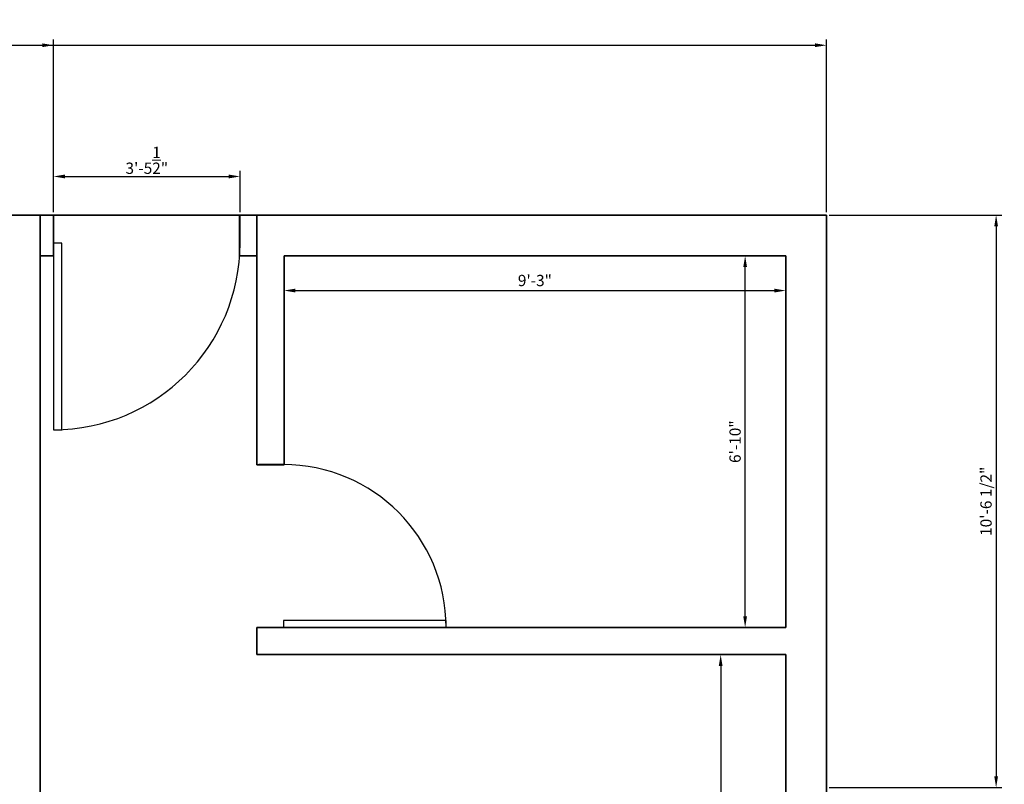
# Model space of a CAD drawing. Units: inches. Extents: x 2025 to 2528, y 1525 to 2336.
# Tile 18 of 18: x 2311 to 2528, y 2167 to 2336. Entities that reach past the tile are written whole.
import ezdxf

# ---------------------------------------------------------------- set-up
doc = ezdxf.new("R2010")
doc.units = ezdxf.units.IN
for name, color, linetype, lineweight in [('A-ANNO-DIMS', 2, 'Continuous', 18), ('A-DOOR', 3, 'Continuous', 25), ('A-WALL', 7, 'Continuous', 35)]:
    doc.layers.add(name, color=color, linetype=linetype, lineweight=lineweight)
doc.styles.get("Standard").update_dxf_attribs({"font": 'arial.ttf'})
doc.dimstyles.new('Copy of ISO-25', dxfattribs={"dimtxt": 2.5, "dimasz": 2.5, "dimexe": 1.25, "dimexo": 0.625, "dimtad": 1, "dimdec": 1, "dimlunit": 4, "dimtxsty": 'Standard', "dimcen": 2.5, "dimadec": 0, "dimazin": 0, "dimtfac": 1, "dimtdec": 1, "dimtmove": 0, "dimatfit": 3, "dimfxl": 1, "dimarcsym": 0})

# ---------------------------------------------------------------- blocks, each defined once
blk = doc.blocks.new('*U2')
for p, q in [((0, 0), (0, 6)), ((40, 0), (40, 6))]:
    blk.add_line(p, q)
blk.add_lwpolyline([(0, 0), (0, -40), (1.75, -40), (1.75, 0)], close=True)
blk.add_arc((0, 0), 40, 270, 0)
blk = doc.blocks.new('*D16')
at = {"layer": 'A-ANNO-DIMS', "color": 0, "lineweight": -2, "transparency": 16777216}
for p, q in [((2369.01, 2282.79), (2369.01, 2274.47)), ((2480.01, 2282.79), (2480.01, 2274.47)), ((2371.51, 2275.72), (2477.51, 2275.72))]:
    blk.add_line(p, q, dxfattribs=at)
at = {"layer": 'A-ANNO-DIMS', "color": 0, "transparency": 16777216}
for points in [[(2371.51, 2276.14), (2371.51, 2275.3), (2369.01, 2275.72)], [(2477.51, 2276.14), (2477.51, 2275.3), (2480.01, 2275.72)]]:
    blk.add_solid(points, dxfattribs=at)
at = {"layer": 'Defpoints', "color": 0, "transparency": 16777216}
for p in [(2369.01, 2283.41), (2480.01, 2283.41), (2480.01, 2275.72)]:
    blk.add_point(p, dxfattribs=at)
at = {"layer": 'A-ANNO-DIMS', "color": 0, "transparency": 16777216, "insert": (2424.51, 2277.62), "char_height": 2.5, "attachment_point": 5}
blk.add_mtext('9\'-3"', dxfattribs=at)
blk = doc.blocks.new('*D17')
at = {"layer": 'A-ANNO-DIMS', "color": 0, "lineweight": -2, "transparency": 16777216}
for p, q in [((2479.39, 2283.41), (2469.78, 2283.41)), ((2471.03, 2203.72), (2471.03, 2280.91)), ((2479.39, 2201.22), (2469.78, 2201.22))]:
    blk.add_line(p, q, dxfattribs=at)
at = {"layer": 'A-ANNO-DIMS', "color": 0, "transparency": 16777216}
for points in [[(2470.61, 2280.91), (2471.45, 2280.91), (2471.03, 2283.41)], [(2470.61, 2203.72), (2471.45, 2203.72), (2471.03, 2201.22)]]:
    blk.add_solid(points, dxfattribs=at)
at = {"layer": 'Defpoints', "color": 0, "transparency": 16777216}
for p in [(2471.03, 2283.41), (2480.01, 2283.41), (2480.01, 2201.22)]:
    blk.add_point(p, dxfattribs=at)
at = {"layer": 'A-ANNO-DIMS', "color": 0, "transparency": 16777216, "insert": (2469.13, 2242.31), "char_height": 2.5, "attachment_point": 5, "rotation": 90}
blk.add_mtext('6\'-10"', dxfattribs=at)
blk = doc.blocks.new('*D18')
at = {"layer": 'A-ANNO-DIMS', "color": 0, "lineweight": -2, "transparency": 16777216}
for p, q in [((2479.39, 2195.22), (2464.37, 2195.22)), ((2465.62, 2192.72), (2465.62, 1943.91)), ((2479.39, 1941.41), (2464.37, 1941.41))]:
    blk.add_line(p, q, dxfattribs=at)
at = {"layer": 'A-ANNO-DIMS', "color": 0, "transparency": 16777216}
for points in [[(2465.2, 2192.72), (2466.03, 2192.72), (2465.62, 2195.22)], [(2465.2, 1943.91), (2466.03, 1943.91), (2465.62, 1941.41)]]:
    blk.add_solid(points, dxfattribs=at)
at = {"layer": 'Defpoints', "color": 0, "transparency": 16777216}
for p in [(2480.01, 2195.22), (2465.62, 1941.41), (2480.01, 1941.41)]:
    blk.add_point(p, dxfattribs=at)
at = {"layer": 'A-ANNO-DIMS', "color": 0, "transparency": 16777216, "insert": (2463.74, 2068.31), "char_height": 2.5, "attachment_point": 5, "rotation": 90}
blk.add_mtext('21\'-2"', dxfattribs=at)
blk = doc.blocks.new('*D20')
at = {"layer": 'A-ANNO-DIMS', "color": 0, "lineweight": -2, "transparency": 16777216}
for p, q in [((2318.01, 2293.04), (2318.01, 2302.2)), ((2320.51, 2300.95), (2356.77, 2300.95)), ((2359.27, 2293.04), (2359.27, 2302.2))]:
    blk.add_line(p, q, dxfattribs=at)
at = {"layer": 'A-ANNO-DIMS', "color": 0, "transparency": 16777216}
for points in [[(2320.51, 2301.37), (2320.51, 2300.53), (2318.01, 2300.95)], [(2356.77, 2301.37), (2356.77, 2300.53), (2359.27, 2300.95)]]:
    blk.add_solid(points, dxfattribs=at)
at = {"layer": 'Defpoints', "color": 0, "transparency": 16777216}
for p in [(2359.27, 2300.95), (2318.01, 2292.41), (2359.27, 2292.41)]:
    blk.add_point(p, dxfattribs=at)
at = {"layer": 'A-ANNO-DIMS', "color": 0, "transparency": 16777216, "insert": (2338.64, 2304.52), "char_height": 2.5, "attachment_point": 5}
blk.add_mtext('3\'-5{\\H1x;\\S1/2;}"', dxfattribs=at)
blk = doc.blocks.new('*D62')
at = {"layer": 'A-ANNO-DIMS', "color": 0, "lineweight": -2, "transparency": 16777216}
for p, q in [((2228.48, 2293.04), (2228.48, 2331.21)), ((2318.01, 2293.04), (2318.01, 2331.21)), ((2230.98, 2329.96), (2315.51, 2329.96))]:
    blk.add_line(p, q, dxfattribs=at)
at = {"layer": 'A-ANNO-DIMS', "color": 0, "transparency": 16777216}
for points in [[(2230.98, 2330.38), (2230.98, 2329.55), (2228.48, 2329.96)], [(2315.51, 2330.38), (2315.51, 2329.55), (2318.01, 2329.96)]]:
    blk.add_solid(points, dxfattribs=at)
at = {"layer": 'Defpoints', "color": 0, "transparency": 16777216}
for p in [(2318.01, 2329.96), (2228.48, 2292.41), (2318.01, 2292.41)]:
    blk.add_point(p, dxfattribs=at)
at = {"layer": 'A-ANNO-DIMS', "color": 0, "transparency": 16777216, "insert": (2273.25, 2331.88), "char_height": 2.5, "attachment_point": 5}
blk.add_mtext('7\'-5 1/2"', dxfattribs=at)
blk = doc.blocks.new('*D63')
at = {"layer": 'A-ANNO-DIMS', "color": 0, "lineweight": -2, "transparency": 16777216}
for p, q in [((2489.64, 2292.41), (2527.81, 2292.41)), ((2526.56, 2289.91), (2526.56, 2168.34)), ((2489.64, 2165.84), (2527.81, 2165.84))]:
    blk.add_line(p, q, dxfattribs=at)
at = {"layer": 'A-ANNO-DIMS', "color": 0, "transparency": 16777216}
for points in [[(2526.15, 2289.91), (2526.98, 2289.91), (2526.56, 2292.41)], [(2526.15, 2168.34), (2526.98, 2168.34), (2526.56, 2165.84)]]:
    blk.add_solid(points, dxfattribs=at)
at = {"layer": 'Defpoints', "color": 0, "transparency": 16777216}
for p in [(2489.01, 2292.41), (2489.01, 2165.84), (2526.56, 2165.84)]:
    blk.add_point(p, dxfattribs=at)
at = {"layer": 'A-ANNO-DIMS', "color": 0, "transparency": 16777216, "insert": (2524.65, 2229.13), "char_height": 2.5, "attachment_point": 5, "rotation": 90}
blk.add_mtext('10\'-6 1/2"', dxfattribs=at)
blk = doc.blocks.new('*D79')
at = {"layer": 'A-ANNO-DIMS', "color": 0, "lineweight": -2, "transparency": 16777216}
for p, q in [((2066.01, 2293.04), (2066.01, 2331.21)), ((2489.01, 2293.04), (2489.01, 2331.21)), ((2068.51, 2329.96), (2486.51, 2329.96))]:
    blk.add_line(p, q, dxfattribs=at)
at = {"layer": 'A-ANNO-DIMS', "color": 0, "transparency": 16777216}
for points in [[(2068.51, 2330.38), (2068.51, 2329.55), (2066.01, 2329.96)], [(2486.51, 2330.38), (2486.51, 2329.55), (2489.01, 2329.96)]]:
    blk.add_solid(points, dxfattribs=at)
at = {"layer": 'Defpoints', "color": 0, "transparency": 16777216}
for p in [(2489.01, 2329.96), (2066.01, 2292.41), (2489.01, 2292.41)]:
    blk.add_point(p, dxfattribs=at)
at = {"layer": 'A-ANNO-DIMS', "color": 0, "transparency": 16777216, "insert": (2277.51, 2331.86), "char_height": 2.5, "attachment_point": 5}
blk.add_mtext('35\'-3"', dxfattribs=at)

msp = doc.modelspace()

# ---------------------------------------------------------------- linework, layer by layer
at = {"layer": 'A-WALL'}
for p, q in [((2252.01, 2292.41), (2312.01, 2292.41)), ((2312.01, 2292.41), (2318.01, 2292.41)), ((2315.01, 2283.41), (2315.01, 2292.41)), ((2318.01, 2292.41), (2366.01, 2292.41)), ((2318.01, 2283.41), (2318.01, 2292.41)), ((2359.13, 2283.41), (2359.13, 2292.41)), ((2363.01, 2283.41), (2363.01, 2292.41)), ((2366.01, 2292.41), (2372.01, 2292.41)), ((2372.01, 2292.41), (2480.01, 2292.41)), ((2480.01, 2292.41), (2489.01, 2292.41)), ((2489.01, 2292.41), (2489.01, 2283.41)), ((2315.01, 2283.41), (2318.01, 2283.41)), ((2315.01, 2115.41), (2315.01, 2283.41)), ((2315.01, 2283.41), (2318.01, 2283.41)), ((2359.13, 2283.41), (2363.01, 2283.41)), ((2363.01, 2283.41), (2359.13, 2283.41)), ((2363.01, 2283.41), (2359.13, 2283.41)), ((2363.01, 2283.41), (2363.01, 2237.22)), ((2369.01, 2283.41), (2372.01, 2283.41)), ((2369.01, 2237.22), (2369.01, 2283.41)), ((2372.01, 2283.41), (2480.01, 2283.41)), ((2480.01, 2283.41), (2480.01, 2201.22)), ((2480.01, 2201.22), (2480.01, 2283.41)), ((2489.01, 1704.41), (2489.01, 2283.41)), ((2363.01, 2237.22), (2369.01, 2237.22)), ((2369.01, 2201.22), (2363.01, 2201.22)), ((2363.01, 2201.22), (2363.01, 2195.22)), ((2480.01, 2201.22), (2369.01, 2201.22)), ((2369.01, 2195.22), (2363.01, 2195.22)), ((2480.01, 2195.22), (2369.01, 2195.22)), ((2480.01, 1713.41), (2480.01, 2195.22)), ((2480.01, 2195.22), (2480.01, 2165.84))]:
    msp.add_line(p, q, dxfattribs=at)

# ---------------------------------------------------------------- block references
at = {"layer": 'A-DOOR', "xscale": 1.031453598570252, "yscale": 1.031453598570252, "zscale": 1.031453598570252}
msp.add_blockref('*U2', (2318.01, 2286.22), dxfattribs=at)
at = {"layer": 'A-DOOR', "xscale": 0.9005889628232303, "yscale": 0.9005889628232303, "zscale": 0.9005889628232303, "rotation": 90}
msp.add_blockref('*U2', (2368.85, 2201.22), dxfattribs=at)

# ---------------------------------------------------------------- dimensions: what is measured, and where the dimension line sits
at = {"layer": 'A-ANNO-DIMS'}
for base, p1, p2, override, picture, middle in [((2318.01, 2329.96), (2228.48, 2292.41), (2318.01, 2292.41), {"dimdec": 1, "dimlfac": 1, "dimrnd": 0, "dimzin": 1, "dimdsep": 46, "dimlunit": 4, "dimfrac": 2}, '*D62', (2273.25, 2331.88)), ((2489.01, 2329.96), (2066.01, 2292.41), (2489.01, 2292.41), {"dimdec": 1, "dimlfac": 1, "dimrnd": 0, "dimzin": 1, "dimdsep": 46, "dimlunit": 4, "dimfrac": 2}, '*D79', (2277.51, 2331.86)), ((2359.27, 2300.95), (2318.01, 2292.41), (2359.27, 2292.41), {"dimclrd": 0, "dimclre": 0, "dimclrt": 0}, '*D20', (2338.64, 2304.52)), ((2480.01, 2275.72), (2369.01, 2283.41), (2480.01, 2283.41), {"dimclrd": 0, "dimclre": 0, "dimclrt": 0}, '*D16', (2424.51, 2277.62))]:
    dim = msp.add_linear_dim(base=base, p1=p1, p2=p2, dimstyle='Copy of ISO-25', override=override, dxfattribs=at)
    dim.commit()
    dim.dimension.update_dxf_attribs({"geometry": picture, "text_midpoint": middle})
for base, p1, p2, override, picture, middle in [((2526.56, 2165.84), (2489.01, 2292.41), (2489.01, 2165.84), {"dimdec": 1, "dimlfac": 1, "dimrnd": 0, "dimzin": 1, "dimdsep": 46, "dimlunit": 4, "dimfrac": 2}, '*D63', (2524.65, 2229.13)), ((2471.03, 2283.41), (2480.01, 2201.22), (2480.01, 2283.41), {"dimclrd": 0, "dimclre": 0, "dimclrt": 0}, '*D17', (2469.13, 2242.31)), ((2465.62, 1941.41), (2480.01, 2195.22), (2480.01, 1941.41), {"dimclrd": 0, "dimclre": 0, "dimclrt": 0}, '*D18', (2463.74, 2068.31))]:
    dim = msp.add_linear_dim(base=base, p1=p1, p2=p2, angle=90, dimstyle='Copy of ISO-25', override=override, dxfattribs=at)
    dim.commit()
    dim.dimension.update_dxf_attribs({"geometry": picture, "text_midpoint": middle})

doc.saveas('drawing.dxf')
